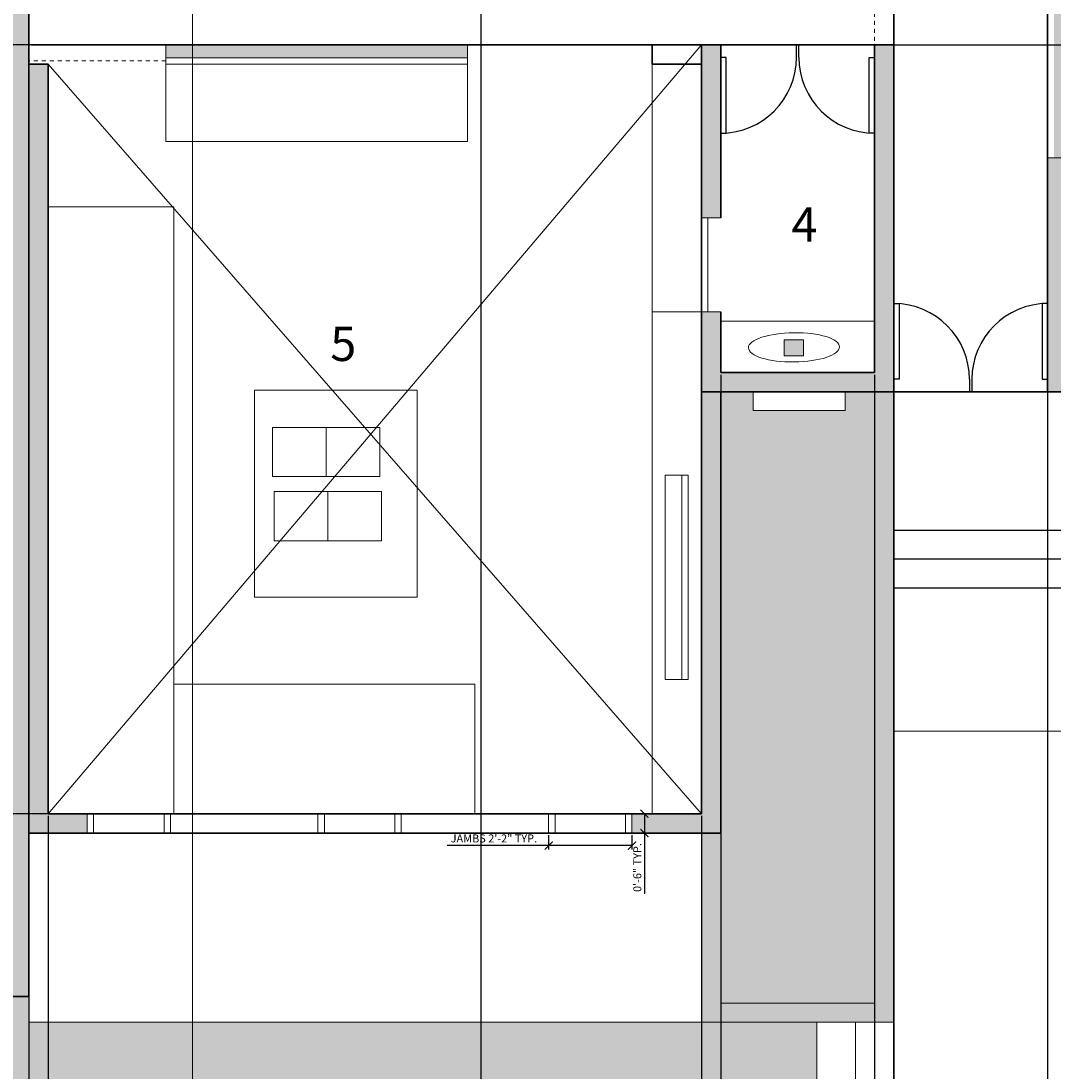
# Model space of a CAD drawing. Units: inches. Extents: x 3122 to 5933, y 1474 to 2995.
# Tile 6 of 12: x 5215 to 5538, y 2032 to 2360. Entities that reach past the tile are written whole.
import ezdxf

# ---------------------------------------------------------------- set-up
doc = ezdxf.new("R2010")
doc.units = ezdxf.units.IN
doc.linetypes.add('JIS_02_1.2', pattern=[2.5, 1.25, -1.25])
for name, color, linetype, lineweight in [('A-ANNO-DIMS', 2, 'Continuous', 18), ('A-ANNO-SYMB', 6, 'Continuous', 18), ('A-AREA-IDEN', 7, 'Continuous', 20), ('A-DETL-PATT', 8, 'Continuous', 13), ('A-DOOR', 4, 'Continuous', 25), ('A-FLOR-CASE', 8, 'Continuous', 18), ('A-FLOR-OPEN', 8, 'Continuous', 13), ('A-FLOR-OVHD', 8, 'JIS_02_1.2', 18), ('A-FLOR-STRS', 7, 'Continuous', 25), ('A-FURN', 8, 'Continuous', 18), ('A-GLAZ', 4, 'Continuous', 18), ('A-WALL', 7, 'Continuous', 35), ('A-WALL-PATT', 7, 'Continuous', 13), ('C-SITE', 8, 'Continuous', 18), ('L-PLNT', 3, 'Continuous', 18), ('L-PLNT-PATT', 94, 'Continuous', 13)]:
    doc.layers.add(name, color=color, linetype=linetype, lineweight=lineweight)
doc.styles.get("Standard").update_dxf_attribs({"font": 'arial.ttf'})
doc.dimstyles.new('ISO-25', dxfattribs={"dimtxt": 2.5, "dimasz": 2.5, "dimexe": 1.25, "dimexo": 0.625, "dimtad": 1, "dimdec": 0, "dimlunit": 3, "dimtxsty": 'Standard', "dimblk": 'ARCHTICK', "dimcen": 2.5, "dimadec": 0, "dimazin": 0, "dimtfac": 1, "dimtdec": 0, "dimtmove": 0, "dimatfit": 3, "dimfxl": 1, "dimarcsym": 0})

# ---------------------------------------------------------------- blocks, each defined once
blk = doc.blocks.new('*U32')
for p, q in [((-600, 0), (-600, -100)), ((0, 0), (0, -100))]:
    blk.add_line(p, q)
blk.add_lwpolyline([(0, 0), (0, 600), (-43.75, 600), (-43.75, 0)], close=True)
blk.add_arc((0, 0), 600, 90, 180)
blk = doc.blocks.new('*U33')
for p, q in [((0, 0), (0, -100)), ((600, 0), (600, -100))]:
    blk.add_line(p, q)
blk.add_lwpolyline([(0, 0), (0, 600), (43.75, 600), (43.75, 0)], close=True)
blk.add_arc((0, 0), 600, 0, 90)
blk = doc.blocks.new('*U34')
for p, q in [((-600, 0), (-600, 100)), ((0, 0), (0, 100))]:
    blk.add_line(p, q)
blk.add_lwpolyline([(0, 0), (0, -600), (-43.75, -600), (-43.75, 0)], close=True)
blk.add_arc((0, 0), 600, 180, 270)
blk = doc.blocks.new('*U35')
for p, q in [((0, 0), (0, 100)), ((600, 0), (600, 100))]:
    blk.add_line(p, q)
blk.add_lwpolyline([(0, 0), (0, -600), (43.75, -600), (43.75, 0)], close=True)
blk.add_arc((0, 0), 600, 270, 0)
blk = doc.blocks.new('WIN-24-PAIRED-JAMBS')
for p, q in [((0, 6), (0, 0)), ((2, 6), (2, 0)), ((24, 6), (24, 0)), ((26, 6), (26, 0))]:
    blk.add_line(p, q)
blk = doc.blocks.new('_ArchTick')
at = {"color": 0, "linetype": 'ByBlock', "const_width": 0.15}
blk.add_lwpolyline([(-0.5, -0.5), (0.5, 0.5)], dxfattribs=at)
blk = doc.blocks.new('*D70')
at = {"layer": 'A-ANNO-DIMS', "color": 0, "lineweight": -2, "transparency": 16777216}
for p, q in [((5380.14, 2106.06), (5380.14, 2101.54)), ((5406.14, 2106.06), (5406.14, 2101.54)), ((5380.14, 2102.79), (5348.49, 2102.79)), ((5406.14, 2102.79), (5380.14, 2102.79))]:
    blk.add_line(p, q, dxfattribs=at)
at = {"layer": 'Defpoints', "color": 0, "transparency": 16777216}
for p in [(5380.14, 2106.69), (5406.14, 2106.69), (5380.14, 2102.79)]:
    blk.add_point(p, dxfattribs=at)
at = {"layer": 'A-ANNO-DIMS', "color": 0, "lineweight": -2, "transparency": 16777216, "xscale": 2.5, "yscale": 2.5, "zscale": 2.5, "rotation": 180}
blk.add_blockref('_ArchTick', (5380.14, 2102.79), dxfattribs=at)
at = {"layer": 'A-ANNO-DIMS', "color": 0, "lineweight": -2, "transparency": 16777216, "xscale": 2.5, "yscale": 2.5, "zscale": 2.5}
blk.add_blockref('_ArchTick', (5406.14, 2102.79), dxfattribs=at)
at = {"layer": 'A-ANNO-DIMS', "color": 0, "transparency": 16777216, "insert": (5363.06, 2104.7), "char_height": 2.5, "attachment_point": 5}
blk.add_mtext('JAMBS 2\'-2" TYP.', dxfattribs=at)
blk = doc.blocks.new('*D71')
at = {"layer": 'A-ANNO-DIMS', "color": 0, "lineweight": -2, "transparency": 16777216}
for p, q in [((5406.77, 2112.69), (5411.29, 2112.69)), ((5410.04, 2112.69), (5410.04, 2106.69)), ((5406.77, 2106.69), (5411.29, 2106.69)), ((5410.04, 2106.69), (5410.04, 2087.7))]:
    blk.add_line(p, q, dxfattribs=at)
at = {"layer": 'Defpoints', "color": 0, "transparency": 16777216}
for p in [(5406.14, 2112.69), (5406.14, 2106.69), (5410.04, 2106.69)]:
    blk.add_point(p, dxfattribs=at)
at = {"layer": 'A-ANNO-DIMS', "color": 0, "lineweight": -2, "transparency": 16777216, "xscale": 2.5, "yscale": 2.5, "zscale": 2.5}
for p, rotation in [((5410.04, 2112.69), 90), ((5410.04, 2106.69), 270)]:
    blk.add_blockref('_ArchTick', p, dxfattribs=dict(at, rotation=rotation))
at = {"layer": 'A-ANNO-DIMS', "color": 0, "transparency": 16777216, "insert": (5408.14, 2095.94), "char_height": 2.5, "attachment_point": 5, "rotation": 90}
blk.add_mtext('0\'-6" TYP.', dxfattribs=at)
blk = doc.blocks.new('*D94')
at = {"layer": 'A-ANNO-DIMS', "color": 0, "lineweight": -2, "transparency": 16777216}
for p, q in [((5064.96, 1916.52), (5064.96, 2990.75)), ((5064.96, 2989.5), (5487.87, 2989.5)), ((5487.87, 1916.52), (5487.87, 2990.75))]:
    blk.add_line(p, q, dxfattribs=at)
at = {"layer": 'Defpoints', "color": 0, "transparency": 16777216}
for p in [(5487.87, 2989.5), (5064.96, 1915.9), (5487.87, 1915.9)]:
    blk.add_point(p, dxfattribs=at)
at = {"layer": 'A-ANNO-DIMS', "color": 0, "lineweight": -2, "transparency": 16777216, "xscale": 2.5, "yscale": 2.5, "zscale": 2.5, "rotation": 180}
blk.add_blockref('_ArchTick', (5064.96, 2989.5), dxfattribs=at)
at = {"layer": 'A-ANNO-DIMS', "color": 0, "lineweight": -2, "transparency": 16777216, "xscale": 2.5, "yscale": 2.5, "zscale": 2.5}
blk.add_blockref('_ArchTick', (5487.87, 2989.5), dxfattribs=at)
at = {"layer": 'A-ANNO-DIMS', "color": 0, "transparency": 16777216, "insert": (5276.42, 2991.41), "char_height": 2.5, "attachment_point": 5}
blk.add_mtext('35\'-3"', dxfattribs=at)
blk = doc.blocks.new('*D103')
at = {"layer": 'A-ANNO-DIMS', "color": 0, "lineweight": -2, "transparency": 16777216}
for p, q in [((5223.96, 2112.06), (5223.96, 1792.93)), ((5427.87, 2112.06), (5427.87, 1792.93)), ((5223.96, 1794.18), (5427.87, 1794.18))]:
    blk.add_line(p, q, dxfattribs=at)
at = {"layer": 'Defpoints', "color": 0, "transparency": 16777216}
for p in [(5223.96, 2112.69), (5427.87, 2112.69), (5427.87, 1794.18)]:
    blk.add_point(p, dxfattribs=at)
at = {"layer": 'A-ANNO-DIMS', "color": 0, "lineweight": -2, "transparency": 16777216, "xscale": 2.5, "yscale": 2.5, "zscale": 2.5, "rotation": 180}
blk.add_blockref('_ArchTick', (5223.96, 1794.18), dxfattribs=at)
at = {"layer": 'A-ANNO-DIMS', "color": 0, "lineweight": -2, "transparency": 16777216, "xscale": 2.5, "yscale": 2.5, "zscale": 2.5}
blk.add_blockref('_ArchTick', (5427.87, 1794.18), dxfattribs=at)
at = {"layer": 'A-ANNO-DIMS', "color": 0, "transparency": 16777216, "insert": (5325.92, 1796.08), "char_height": 2.5, "attachment_point": 5}
blk.add_mtext('17\'-0"', dxfattribs=at)
blk = doc.blocks.new('*D104')
at = {"layer": 'A-ANNO-DIMS', "color": 0, "lineweight": -2, "transparency": 16777216}
for p, q in [((5427.24, 2352.69), (4920.36, 2352.69)), ((4921.61, 2112.69), (4921.61, 2352.69)), ((5427.24, 2112.69), (4920.36, 2112.69))]:
    blk.add_line(p, q, dxfattribs=at)
at = {"layer": 'Defpoints', "color": 0, "transparency": 16777216}
for p in [(4921.61, 2352.69), (5427.87, 2352.69), (5427.87, 2112.69)]:
    blk.add_point(p, dxfattribs=at)
at = {"layer": 'A-ANNO-DIMS', "color": 0, "lineweight": -2, "transparency": 16777216, "xscale": 2.5, "yscale": 2.5, "zscale": 2.5}
for p, rotation in [((4921.61, 2352.69), 90), ((4921.61, 2112.69), 270)]:
    blk.add_blockref('_ArchTick', p, dxfattribs=dict(at, rotation=rotation))
at = {"layer": 'A-ANNO-DIMS', "color": 0, "transparency": 16777216, "insert": (4919.71, 2232.69), "char_height": 2.5, "attachment_point": 5, "rotation": 90}
blk.add_mtext('20\'-0"', dxfattribs=at)
blk = doc.blocks.new('*D105')
at = {"layer": 'A-ANNO-DIMS', "color": 0, "lineweight": -2, "transparency": 16777216}
for p, q in [((5433.87, 2249.76), (5433.87, 1792.93)), ((5481.87, 2249.76), (5481.87, 1792.93)), ((5433.87, 1794.18), (5481.87, 1794.18))]:
    blk.add_line(p, q, dxfattribs=at)
at = {"layer": 'Defpoints', "color": 0, "transparency": 16777216}
for p in [(5433.87, 2250.39), (5481.87, 2250.39), (5481.87, 1794.18)]:
    blk.add_point(p, dxfattribs=at)
at = {"layer": 'A-ANNO-DIMS', "color": 0, "lineweight": -2, "transparency": 16777216, "xscale": 2.5, "yscale": 2.5, "zscale": 2.5, "rotation": 180}
blk.add_blockref('_ArchTick', (5433.87, 1794.18), dxfattribs=at)
at = {"layer": 'A-ANNO-DIMS', "color": 0, "lineweight": -2, "transparency": 16777216, "xscale": 2.5, "yscale": 2.5, "zscale": 2.5}
blk.add_blockref('_ArchTick', (5481.87, 1794.18), dxfattribs=at)
at = {"layer": 'A-ANNO-DIMS', "color": 0, "transparency": 16777216, "insert": (5457.87, 1796.08), "char_height": 2.5, "attachment_point": 5}
blk.add_mtext('4\'-0"', dxfattribs=at)
blk = doc.blocks.new('*D108')
at = {"layer": 'A-ANNO-DIMS', "color": 0, "lineweight": -2, "transparency": 16777216}
for p, q in [((5178.96, 2643.06), (5178.96, 1792.93)), ((5358.96, 2643.06), (5358.96, 1792.93)), ((5178.96, 1794.18), (5358.96, 1794.18))]:
    blk.add_line(p, q, dxfattribs=at)
at = {"layer": 'Defpoints', "color": 0, "transparency": 16777216}
for p in [(5178.96, 2643.69), (5358.96, 2643.69), (5358.96, 1794.18)]:
    blk.add_point(p, dxfattribs=at)
at = {"layer": 'A-ANNO-DIMS', "color": 0, "lineweight": -2, "transparency": 16777216, "xscale": 2.5, "yscale": 2.5, "zscale": 2.5, "rotation": 180}
blk.add_blockref('_ArchTick', (5178.96, 1794.18), dxfattribs=at)
at = {"layer": 'A-ANNO-DIMS', "color": 0, "lineweight": -2, "transparency": 16777216, "xscale": 2.5, "yscale": 2.5, "zscale": 2.5}
blk.add_blockref('_ArchTick', (5358.96, 1794.18), dxfattribs=at)
at = {"layer": 'A-ANNO-DIMS', "color": 0, "transparency": 16777216, "insert": (5268.96, 1796.08), "char_height": 2.5, "attachment_point": 5}
blk.add_mtext('15\'-0"', dxfattribs=at)
blk = doc.blocks.new('*D110')
at = {"layer": 'A-ANNO-DIMS', "color": 0, "lineweight": -2, "transparency": 16777216}
for p, q in [((5487.87, 2643.06), (5487.87, 1792.93)), ((5670.96, 2643.06), (5670.96, 1792.93)), ((5487.87, 1794.18), (5670.96, 1794.18))]:
    blk.add_line(p, q, dxfattribs=at)
at = {"layer": 'Defpoints', "color": 0, "transparency": 16777216}
for p in [(5487.87, 2643.69), (5670.96, 2643.69), (5670.96, 1794.18)]:
    blk.add_point(p, dxfattribs=at)
at = {"layer": 'A-ANNO-DIMS', "color": 0, "lineweight": -2, "transparency": 16777216, "xscale": 2.5, "yscale": 2.5, "zscale": 2.5, "rotation": 180}
blk.add_blockref('_ArchTick', (5487.87, 1794.18), dxfattribs=at)
at = {"layer": 'A-ANNO-DIMS', "color": 0, "lineweight": -2, "transparency": 16777216, "xscale": 2.5, "yscale": 2.5, "zscale": 2.5}
blk.add_blockref('_ArchTick', (5670.96, 1794.18), dxfattribs=at)
at = {"layer": 'A-ANNO-DIMS', "color": 0, "transparency": 16777216, "insert": (5579.42, 1796.09), "char_height": 2.5, "attachment_point": 5}
blk.add_mtext('15\'-3"', dxfattribs=at)
blk = doc.blocks.new('*D115')
at = {"layer": 'A-ANNO-DIMS', "color": 0, "lineweight": -2, "transparency": 16777216}
for p, q in [((5217.96, 2532.06), (5217.96, 1792.93)), ((5535.87, 2532.06), (5535.87, 1792.93)), ((5217.96, 1794.18), (5535.87, 1794.18))]:
    blk.add_line(p, q, dxfattribs=at)
at = {"layer": 'Defpoints', "color": 0, "transparency": 16777216}
for p in [(5217.96, 2532.69), (5535.87, 2532.69), (5535.87, 1794.18)]:
    blk.add_point(p, dxfattribs=at)
at = {"layer": 'A-ANNO-DIMS', "color": 0, "lineweight": -2, "transparency": 16777216, "xscale": 2.5, "yscale": 2.5, "zscale": 2.5, "rotation": 180}
blk.add_blockref('_ArchTick', (5217.96, 1794.18), dxfattribs=at)
at = {"layer": 'A-ANNO-DIMS', "color": 0, "lineweight": -2, "transparency": 16777216, "xscale": 2.5, "yscale": 2.5, "zscale": 2.5}
blk.add_blockref('_ArchTick', (5535.87, 1794.18), dxfattribs=at)
at = {"layer": 'A-ANNO-DIMS', "color": 0, "transparency": 16777216, "insert": (5376.92, 1796.08), "char_height": 2.5, "attachment_point": 5}
blk.add_mtext('26\'-6"', dxfattribs=at)
blk = doc.blocks.new('*D116')
at = {"layer": 'A-ANNO-DIMS', "color": 0, "lineweight": -2, "transparency": 16777216}
for p, q in [((5218.59, 2532.69), (5931.98, 2532.69)), ((5930.73, 2352.69), (5930.73, 2532.69)), ((5218.59, 2352.69), (5931.98, 2352.69))]:
    blk.add_line(p, q, dxfattribs=at)
at = {"layer": 'Defpoints', "color": 0, "transparency": 16777216}
for p in [(5217.96, 2532.69), (5930.73, 2532.69), (5217.96, 2352.69)]:
    blk.add_point(p, dxfattribs=at)
at = {"layer": 'A-ANNO-DIMS', "color": 0, "lineweight": -2, "transparency": 16777216, "xscale": 2.5, "yscale": 2.5, "zscale": 2.5}
for p, rotation in [((5930.73, 2532.69), 90), ((5930.73, 2352.69), 270)]:
    blk.add_blockref('_ArchTick', p, dxfattribs=dict(at, rotation=rotation))
at = {"layer": 'A-ANNO-DIMS', "color": 0, "transparency": 16777216, "insert": (5928.83, 2442.69), "char_height": 2.5, "attachment_point": 5, "rotation": 90}
blk.add_mtext('15\'-0"', dxfattribs=at)
blk = doc.blocks.new('*D117')
at = {"layer": 'A-ANNO-DIMS', "color": 0, "lineweight": -2, "transparency": 16777216}
for p, q in [((5488.49, 2244.39), (5931.98, 2244.39)), ((5930.73, 1915.9), (5930.73, 2244.39)), ((5488.49, 1915.9), (5931.98, 1915.9))]:
    blk.add_line(p, q, dxfattribs=at)
at = {"layer": 'Defpoints', "color": 0, "transparency": 16777216}
for p in [(5487.87, 2244.39), (5930.73, 2244.39), (5487.87, 1915.9)]:
    blk.add_point(p, dxfattribs=at)
at = {"layer": 'A-ANNO-DIMS', "color": 0, "lineweight": -2, "transparency": 16777216, "xscale": 2.5, "yscale": 2.5, "zscale": 2.5}
for p, rotation in [((5930.73, 2244.39), 90), ((5930.73, 1915.9), 270)]:
    blk.add_blockref('_ArchTick', p, dxfattribs=dict(at, rotation=rotation))
at = {"layer": 'A-ANNO-DIMS', "color": 0, "transparency": 16777216, "insert": (5928.81, 2080.14), "char_height": 2.5, "attachment_point": 5, "rotation": 90}
blk.add_mtext('27\'-4 1/2"', dxfattribs=at)
blk = doc.blocks.new('*D119')
at = {"layer": 'A-ANNO-DIMS', "color": 0, "lineweight": -2, "transparency": 16777216}
for p, q in [((5487.87, 2247.7), (5487.87, 1792.93)), ((5535.87, 2247.7), (5535.87, 1792.93)), ((5487.87, 1794.18), (5535.87, 1794.18))]:
    blk.add_line(p, q, dxfattribs=at)
at = {"layer": 'Defpoints', "color": 0, "transparency": 16777216}
for p in [(5487.87, 2248.32), (5535.87, 2248.32), (5535.87, 1794.18)]:
    blk.add_point(p, dxfattribs=at)
at = {"layer": 'A-ANNO-DIMS', "color": 0, "lineweight": -2, "transparency": 16777216, "xscale": 2.5, "yscale": 2.5, "zscale": 2.5, "rotation": 180}
blk.add_blockref('_ArchTick', (5487.87, 1794.18), dxfattribs=at)
at = {"layer": 'A-ANNO-DIMS', "color": 0, "lineweight": -2, "transparency": 16777216, "xscale": 2.5, "yscale": 2.5, "zscale": 2.5}
blk.add_blockref('_ArchTick', (5535.87, 1794.18), dxfattribs=at)
at = {"layer": 'A-ANNO-DIMS', "color": 0, "transparency": 16777216, "insert": (5511.87, 1796.08), "char_height": 2.5, "attachment_point": 5}
blk.add_mtext('4\'-0"', dxfattribs=at)

msp = doc.modelspace()

# ---------------------------------------------------------------- hatches: boundary and pattern name
at = {"layer": 'A-DETL-PATT'}
h = msp.add_hatch(color=256, dxfattribs=at)
h.dxf.hatch_style = 1
h.paths.add_polyline_path([(5459.7, 2260.67), (5453.68, 2260.67), (5453.68, 2255.61), (5459.7, 2255.61)])
at = {"layer": 'A-WALL-PATT'}
h = msp.add_hatch(color=256, dxfattribs=at)
h.dxf.hatch_style = 1
h.paths.add_polyline_path([(5073.96, 2454.69), (5101.59, 2454.69), (5101.59, 2459.69), (5101.59, 2463.69), (5073.96, 2463.69), (5073.96, 2634.69), (5169.96, 2634.69), (5364.96, 2634.69), (5364.96, 2643.69), (5364.96, 2667.06), (5358.96, 2667.06), (5358.96, 2643.69), (5178.96, 2643.69), (5178.96, 2655.69), (5169.96, 2655.69), (5169.96, 2643.69), (5073.96, 2643.69), (5073.96, 2745.9), (5124.13, 2745.9), (5124.13, 2754.9), (5073.96, 2754.9), (5073.96, 2866.9), (5169.96, 2866.9), (5169.96, 2818.9), (5169.96, 2812.9), (5169.96, 2754.9), (5154.13, 2754.9), (5154.13, 2745.9), (5169.96, 2745.9), (5169.96, 2691.69), (5178.96, 2691.69), (5178.96, 2812.9), (5178.96, 2818.9), (5178.96, 2875.9), (5064.96, 2875.9), (5064.96, 2055.71), (5217.96, 2055.71), (5217.96, 2464.19), (5212.96, 2464.19), (5212.96, 2463.69), (5148.19, 2463.69), (5148.19, 2459.69), (5148.19, 2454.69), (5158.96, 2454.69), (5158.96, 2450.72), (5156.04, 2450.72), (5156.04, 2447.72), (5158.96, 2447.72), (5158.96, 2425.1), (5164.96, 2425.1), (5164.96, 2447.72), (5167.71, 2447.72), (5167.71, 2450.72), (5164.96, 2450.72), (5164.96, 2454.69), (5212.96, 2454.69), (5212.96, 2064.71), (5073.96, 2064.71), (5073.96, 2322.69), (5158.96, 2322.69), (5164.96, 2322.69), (5164.96, 2328.69), (5158.96, 2328.69), (5073.96, 2328.69)])
h = msp.add_hatch(color=256, dxfattribs=at)
h.dxf.hatch_style = 1
h.paths.add_polyline_path([(5536.42, 2643.69), (5487.87, 2643.69), (5487.87, 2667.06), (5485.81, 2667.06), (5481.87, 2667.06), (5481.87, 2643.69), (5481.87, 2590.35), (5487.87, 2590.35), (5487.87, 2634.69), (5524.65, 2634.69), (5524.65, 2538.69), (5487.87, 2538.69), (5487.87, 2554.35), (5481.87, 2554.35), (5481.87, 2532.69), (5524.65, 2532.69), (5658.65, 2532.69), (5718.65, 2532.69), (5718.65, 2501.93), (5724.65, 2501.93), (5724.65, 2549.4), (5718.65, 2549.4), (5718.65, 2538.69), (5658.65, 2538.69), (5658.65, 2573.57), (5658.59, 2573.63), (5654.65, 2573.63), (5654.65, 2538.69), (5594.65, 2538.69), (5594.65, 2573.57), (5594.59, 2573.63), (5590.65, 2573.63), (5590.65, 2538.69), (5530.65, 2538.69), (5530.65, 2634.69), (5536.42, 2634.69)])
h.paths.add_polyline_path([(5735.69, 2643.69), (5679.96, 2643.69), (5679.96, 2710.77), (5720.44, 2710.77), (5720.44, 2687.32), (5737.79, 2687.32), (5737.79, 2692.32), (5725.44, 2692.32), (5725.44, 2715.77), (5679.96, 2715.77), (5679.96, 2866.9), (5775.96, 2866.9), (5775.96, 2692.32), (5773.79, 2692.32), (5773.79, 2687.32), (5775.96, 2687.32), (5775.96, 2643.69), (5775.96, 2591.85), (5784.96, 2591.85), (5784.96, 2875.9), (5670.96, 2875.9), (5670.96, 2818.9), (5412.4, 2818.9), (5412.4, 2812.9), (5460.96, 2812.9), (5460.96, 2719.12), (5404.54, 2719.12), (5404.54, 2713.12), (5466.96, 2713.12), (5481.87, 2713.12), (5481.87, 2703.06), (5487.87, 2703.06), (5487.87, 2719.12), (5466.96, 2719.12), (5466.96, 2812.9), (5670.96, 2812.9), (5670.96, 2643.69), (5572.42, 2643.69), (5572.42, 2634.69), (5718.65, 2634.69), (5718.65, 2549.4), (5724.65, 2549.4), (5724.65, 2591.85), (5739.96, 2591.85), (5739.96, 2596.85), (5724.65, 2596.85), (5724.65, 2634.69), (5735.69, 2634.69)])
h.paths.add_polyline_path([(5594.65, 2634.69), (5590.65, 2634.69), (5590.65, 2603.63), (5594.65, 2603.63)], flags=17)
h.paths.add_polyline_path([(5724.65, 2441.93), (5718.65, 2441.93), (5718.65, 2336.51), (5724.65, 2336.51)])
h.paths.add_polyline_path([(5724.65, 2276.51), (5718.65, 2276.51), (5718.65, 2250.49), (5713.26, 2250.49), (5713.26, 2244.39), (5724.65, 2244.39)])
h.paths.add_polyline_path([(5689.26, 2250.49), (5540.87, 2250.49), (5540.87, 2317.46), (5535.87, 2317.46), (5535.87, 2244.39), (5689.26, 2244.39)])
h.paths.add_polyline_path([(5540.87, 2532.69), (5535.87, 2532.69), (5535.87, 2472.78), (5540.87, 2472.78)])
h.paths.add_polyline_path([(5540.87, 2472.78), (5537.87, 2472.78), (5537.87, 2346.69), (5537.87, 2317.46), (5540.87, 2317.46)])
h = msp.add_hatch(color=256, dxfattribs=at)
h.dxf.hatch_style = 1
h.paths.add_polyline_path([(5354.78, 2352.69), (5260.69, 2352.69), (5260.69, 2348.69), (5354.78, 2348.69)])
h.paths.add_polyline_path([(5223.96, 2346.69), (5217.96, 2346.69), (5217.96, 2106.69), (5236.14, 2106.69), (5236.14, 2112.69), (5223.96, 2112.69)])
h = msp.add_hatch(color=256, dxfattribs=at)
h.dxf.hatch_style = 1
h.paths.add_polyline_path([(5433.87, 2346.69), (5433.87, 2352.69), (5427.87, 2352.69), (5427.87, 2298.69), (5433.87, 2298.69)], flags=17)
h.paths.add_polyline_path([(5487.87, 2352.69), (5481.87, 2352.69), (5481.87, 2346.69), (5481.87, 2269.32), (5481.87, 2250.39), (5433.87, 2250.39), (5433.87, 2269.32), (5427.87, 2269.32), (5427.87, 2244.39), (5487.87, 2244.39)])
h.paths.add_polyline_path([(5433.87, 2244.39), (5427.87, 2244.39), (5427.87, 2112.69), (5406.14, 2112.69), (5406.14, 2106.69), (5433.87, 2106.69)])
at = {"layer": 'L-PLNT-PATT'}
h = msp.add_hatch(color=256, dxfattribs=at)
h.dxf.hatch_style = 1
h.paths.add_polyline_path([(5487.87, 2244.39), (5481.87, 2244.39), (5481.87, 2053.66), (5433.87, 2053.66), (5433.87, 2106.69), (5427.87, 2106.69), (5427.87, 2047.66), (5487.87, 2047.66)])
h = msp.add_hatch(dxfattribs=at)
h.set_pattern_fill('GRASS', color=256, scale=0.1)
h.paths.add_polyline_path([(5481.87, 2244.39), (5472.74, 2244.39), (5472.74, 2238.61), (5444, 2238.61), (5444, 2244.39), (5433.87, 2244.39), (5433.87, 2106.69), (5433.87, 2053.66), (5481.87, 2053.66)])
h = msp.add_hatch(dxfattribs=at)
h.set_pattern_fill('GRASS', color=256, scale=0.1)
h.paths.add_polyline_path([(5463.87, 2047.66), (5427.87, 2047.66), (5217.96, 2047.66), (5217.96, 2055.71), (5092.96, 2055.71), (5092.96, 1919.9), (5463.87, 1919.9)])

# ---------------------------------------------------------------- linework, layer by layer
at = {"layer": 'A-ANNO-SYMB'}
msp.add_line((5268.96, 2933.31), (5268.96, 1850.37), dxfattribs=at)
at = {"layer": 'A-FLOR-CASE'}
for p, q in [((5412.41, 2269.32), (5412.41, 2352.69)), ((5427.87, 2269.32), (5412.41, 2269.32)), ((5412.41, 2269.32), (5412.41, 2112.69)), ((5433.87, 2266.42), (5481.87, 2266.42)), ((5416.48, 2218.35), (5423.71, 2218.35)), ((5416.48, 2154.59), (5416.48, 2218.35)), ((5421.71, 2218.35), (5421.71, 2154.59)), ((5423.71, 2218.35), (5423.71, 2154.59)), ((5423.71, 2154.59), (5416.48, 2154.59))]:
    msp.add_line(p, q, dxfattribs=at)
msp.add_lwpolyline([(5453.68, 2260.67), (5459.7, 2260.67), (5459.7, 2255.61), (5453.68, 2255.61)], close=True, dxfattribs=at)
msp.add_ellipse((5456.72, 2258.29), major_axis=(14.22, 0.15), ratio=0.321498, dxfattribs=at)
at = {"layer": 'A-FLOR-OPEN'}
for p, q in [((5427.87, 2352.69), (5223.96, 2112.69)), ((5223.96, 2346.69), (5427.87, 2112.69))]:
    msp.add_line(p, q, dxfattribs=at)
at = {"layer": 'A-FLOR-OVHD'}
for p, q in [((5481.87, 2532.69), (5481.87, 2352.69)), ((5487.87, 2532.69), (5487.87, 2352.69)), ((5260.69, 2352.69), (5217.96, 2352.69)), ((5412.41, 2352.69), (5354.78, 2352.69)), ((5260.69, 2347.69), (5217.96, 2347.69))]:
    msp.add_line(p, q, dxfattribs=at)
at = {"layer": 'A-FLOR-STRS'}
for p, q in [((5655.13, 2201.13), (5487.87, 2201.13)), ((5664.13, 2192.13), (5487.87, 2192.13)), ((5673.13, 2183.13), (5487.87, 2183.13))]:
    msp.add_line(p, q, dxfattribs=at)
at = {"layer": 'A-FURN'}
for p, q in [((5260.69, 2346.69), (5260.69, 2322.58)), ((5354.78, 2322.58), (5354.78, 2346.69)), ((5260.69, 2322.58), (5354.78, 2322.58)), ((5223.96, 2302.12), (5263.18, 2302.12)), ((5263.18, 2302.12), (5263.18, 2112.69)), ((5263.18, 2153.12), (5357.1, 2153.12)), ((5357.1, 2153.12), (5357.1, 2112.69))]:
    msp.add_line(p, q, dxfattribs=at)
for points in [[(5288.29, 2244.92), (5339.09, 2244.92), (5339.09, 2180.28), (5288.29, 2180.28)], [(5293.97, 2233.28), (5310.69, 2233.28), (5310.69, 2217.94), (5293.97, 2217.94)], [(5310.69, 2233.28), (5327.41, 2233.28), (5327.41, 2217.94), (5310.69, 2217.94)], [(5294.52, 2213.29), (5311.24, 2213.29), (5311.24, 2197.95), (5294.52, 2197.95)], [(5311.24, 2213.29), (5327.96, 2213.29), (5327.96, 2197.95), (5311.24, 2197.95)]]:
    msp.add_lwpolyline(points, close=True, dxfattribs=at)
at = {"layer": 'A-GLAZ'}
for p, q in [((5260.69, 2352.69), (5354.78, 2352.69)), ((5260.69, 2352.69), (5260.69, 2346.69)), ((5354.78, 2346.69), (5354.78, 2352.69)), ((5260.69, 2348.69), (5354.78, 2348.69)), ((5260.69, 2346.69), (5354.78, 2346.69)), ((5540.87, 2317.46), (5535.87, 2317.46)), ((5433.87, 2298.69), (5427.87, 2298.69)), ((5429.87, 2298.69), (5429.87, 2269.32)), ((5427.87, 2269.32), (5433.87, 2269.32))]:
    msp.add_line(p, q, dxfattribs=at)
at = {"layer": 'A-WALL'}
for p, q in [((5535.87, 2346.69), (5535.87, 2532.69)), ((5217.96, 2464.19), (5217.96, 2055.71)), ((5412.41, 2346.69), (5412.41, 2352.69)), ((5412.41, 2352.69), (5433.87, 2352.69)), ((5427.87, 2352.69), (5427.87, 2269.32)), ((5433.87, 2352.69), (5433.87, 2346.69)), ((5433.87, 2352.69), (5481.87, 2352.69)), ((5481.87, 2346.69), (5481.87, 2352.69)), ((5481.87, 2352.69), (5487.87, 2352.69)), ((5487.87, 2352.69), (5487.87, 2244.39)), ((5217.96, 2346.69), (5223.96, 2346.69)), ((5223.96, 2346.69), (5223.96, 2112.69)), ((5412.41, 2346.69), (5427.87, 2346.69)), ((5433.87, 2346.69), (5433.87, 2298.69)), ((5481.87, 2346.69), (5481.87, 2269.32)), ((5535.87, 2346.69), (5535.87, 2244.39)), ((5427.87, 2269.32), (5427.87, 2244.39)), ((5433.87, 2269.32), (5433.87, 2250.39)), ((5481.87, 2250.39), (5481.87, 2269.32)), ((5433.87, 2250.39), (5481.87, 2250.39)), ((5427.87, 2244.39), (5487.87, 2244.39)), ((5427.87, 2244.39), (5427.87, 2112.69)), ((5433.87, 2244.39), (5433.87, 2106.69)), ((5487.87, 2244.39), (5535.87, 2244.39)), ((5535.87, 2244.39), (5724.65, 2244.39)), ((5223.96, 2112.69), (5427.87, 2112.69)), ((5217.96, 2106.69), (5433.87, 2106.69)), ((5217.96, 2055.71), (5064.96, 2055.71))]:
    msp.add_line(p, q, dxfattribs=at)
at = {"layer": 'C-SITE'}
for p, q in [((5724.65, 2138.47), (5487.87, 2138.47)), ((5217.96, 2047.66), (5217.96, 2055.71)), ((5427.87, 2047.66), (5217.96, 2047.66))]:
    msp.add_line(p, q, dxfattribs=at)
at = {"layer": 'L-PLNT'}
for p, q in [((5444, 2244.39), (5444, 2238.61)), ((5472.74, 2238.61), (5472.74, 2244.39)), ((5481.87, 2244.39), (5481.87, 2053.66)), ((5487.87, 2244.39), (5487.87, 2047.66)), ((5444, 2238.61), (5472.74, 2238.61)), ((5427.87, 2047.66), (5427.87, 2106.69)), ((5433.87, 2053.66), (5433.87, 2106.69)), ((5481.87, 2053.66), (5433.87, 2053.66)), ((5487.87, 2047.66), (5427.87, 2047.66)), ((5463.87, 2047.66), (5463.87, 1919.9)), ((5475.87, 2047.66), (5475.87, 1968.97)), ((5487.87, 2047.66), (5487.87, 1919.9))]:
    msp.add_line(p, q, dxfattribs=at)

# ---------------------------------------------------------------- block references
at = {"layer": 'A-DOOR', "xscale": 0.0393700787401575, "yscale": 0.0393700787401575, "zscale": 0.0393700787401575}
for name, p in [('*U35', (5433.87, 2348.75)), ('*U34', (5481.87, 2348.75)), ('*U33', (5487.87, 2248.32)), ('*U32', (5535.87, 2248.32))]:
    msp.add_blockref(name, p, dxfattribs=at)
at = {"layer": 'A-GLAZ'}
msp.add_blockref('WIN-24-PAIRED-JAMBS', (5236.14, 2106.69), dxfattribs=at)
at = {"layer": 'A-GLAZ', "rotation": 180}
for p in [(5334.14, 2112.69), (5406.14, 2112.69)]:
    msp.add_blockref('WIN-24-PAIRED-JAMBS', p, dxfattribs=at)

# ---------------------------------------------------------------- texts
at = {"layer": 'A-AREA-IDEN'}
for s, p in [('4', (5455.93, 2291.27)), ('5', (5312, 2254.04))]:
    msp.add_text(s, height=10.72, rotation=0.0333, dxfattribs=at).set_placement(p)

# ---------------------------------------------------------------- dimensions: what is measured, and where the dimension line sits
at = {"layer": 'A-ANNO-DIMS'}
for base, p1, p2, picture, middle in [((5487.87, 2989.5), (5064.96, 1915.9), (5487.87, 1915.9), '*D94', (5276.42, 2991.41)), ((5358.96, 1794.18), (5178.96, 2643.69), (5358.96, 2643.69), '*D108', (5268.96, 1796.08)), ((5670.96, 1794.18), (5487.87, 2643.69), (5670.96, 2643.69), '*D110', (5579.42, 1796.09)), ((5535.87, 1794.18), (5217.96, 2532.69), (5535.87, 2532.69), '*D115', (5376.92, 1796.08)), ((5481.87, 1794.18), (5433.87, 2250.39), (5481.87, 2250.39), '*D105', (5457.87, 1796.08)), ((5535.87, 1794.18), (5487.87, 2248.32), (5535.87, 2248.32), '*D119', (5511.87, 1796.08)), ((5427.87, 1794.18), (5223.96, 2112.69), (5427.87, 2112.69), '*D103', (5325.92, 1796.08))]:
    dim = msp.add_linear_dim(base=base, p1=p1, p2=p2, dimstyle='ISO-25', override={"dimdec": 1, "dimlfac": 1, "dimrnd": 0, "dimzin": 1, "dimdsep": 46, "dimlunit": 4, "dimfrac": 2}, dxfattribs=at)
    dim.commit()
    dim.dimension.update_dxf_attribs({"geometry": picture, "text_midpoint": middle})
for base, p1, p2, picture, middle in [((5930.73, 2532.69), (5217.96, 2352.69), (5217.96, 2532.69), '*D116', (5928.83, 2442.69)), ((4921.61, 2352.69), (5427.87, 2112.69), (5427.87, 2352.69), '*D104', (4919.71, 2232.69)), ((5930.73, 2244.39), (5487.87, 1915.9), (5487.87, 2244.39), '*D117', (5928.81, 2080.14))]:
    dim = msp.add_linear_dim(base=base, p1=p1, p2=p2, angle=90, dimstyle='ISO-25', override={"dimdec": 1, "dimlfac": 1, "dimrnd": 0, "dimzin": 1, "dimdsep": 46, "dimlunit": 4, "dimfrac": 2}, dxfattribs=at)
    dim.commit()
    dim.dimension.update_dxf_attribs({"geometry": picture, "text_midpoint": middle})
for base, p1, p2, angle, text, picture, middle in [((5410.04, 2106.69), (5406.14, 2112.69), (5406.14, 2106.69), 270, '<> TYP.', '*D71', (5408.14, 2095.94)), ((5380.14, 2102.79), (5406.14, 2106.69), (5380.14, 2106.69), 180, 'JAMBS <> TYP.', '*D70', (5363.06, 2104.7))]:
    dim = msp.add_linear_dim(base=base, p1=p1, p2=p2, angle=angle, text=text, dimstyle='ISO-25', override={"dimdec": 1, "dimlfac": 1, "dimrnd": 0, "dimzin": 1, "dimdsep": 46, "dimlunit": 4, "dimfrac": 2}, dxfattribs=at)
    dim.commit()
    dim.dimension.update_dxf_attribs({"geometry": picture, "text_midpoint": middle})

doc.saveas('drawing.dxf')
